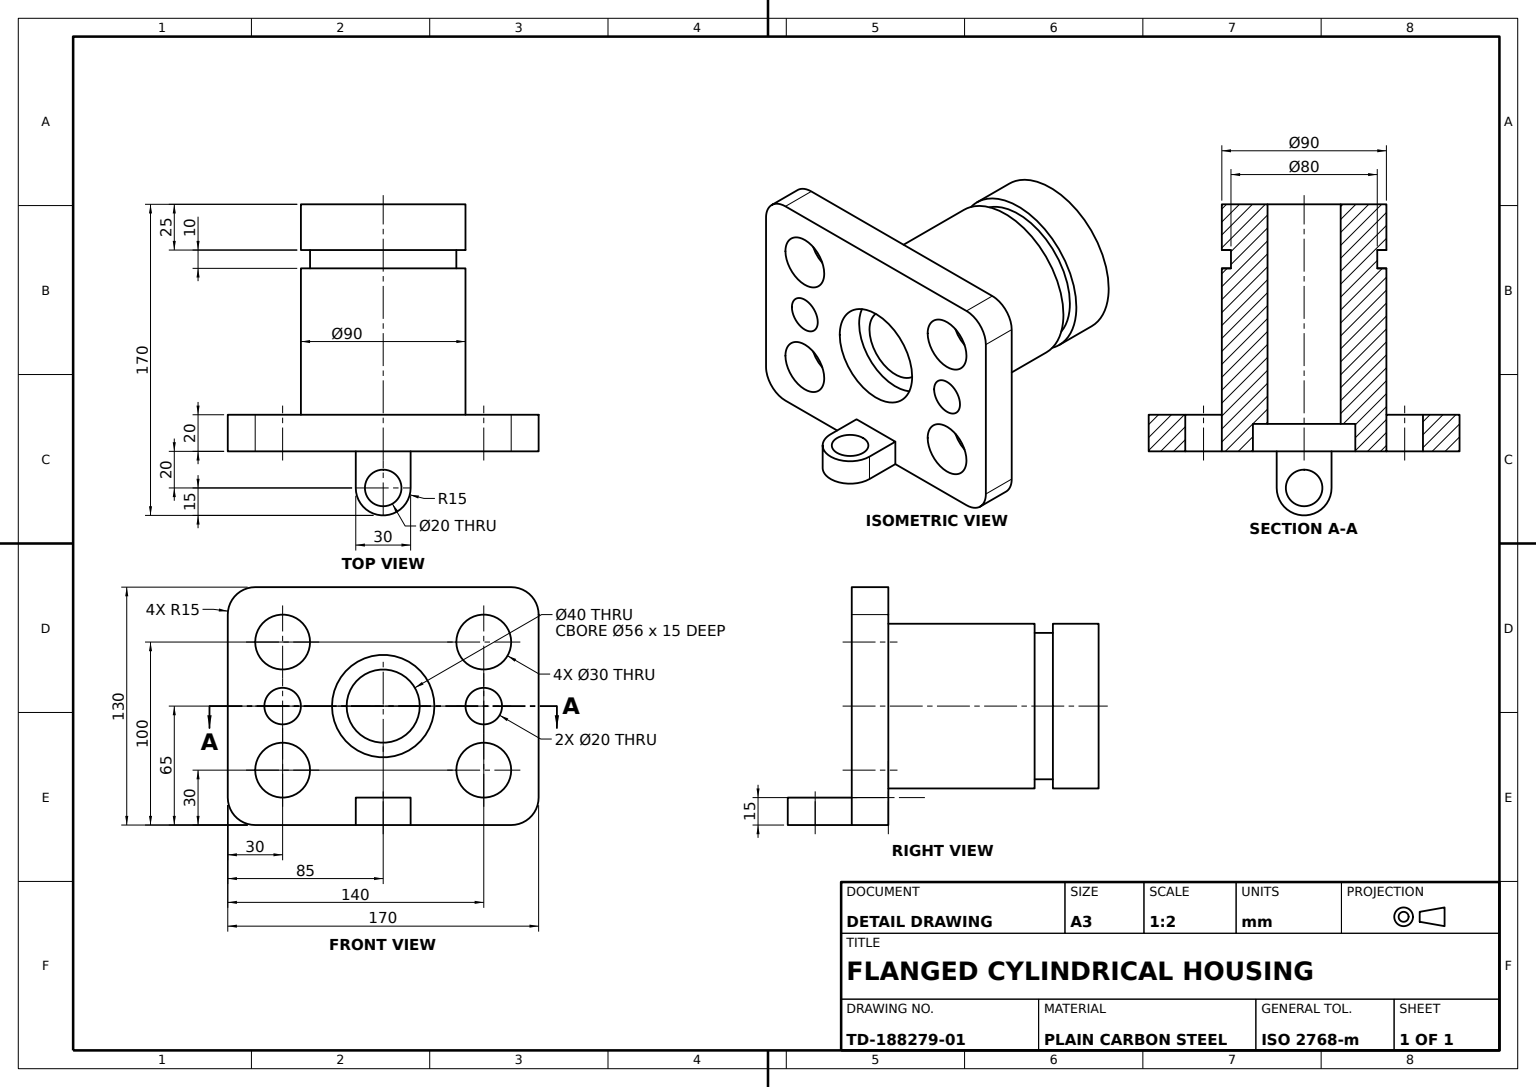
from build123d import *

# Parameters (mm, degrees)
COLUMN_BASE_SKETCH_R    = 45
COLUMN_BASE_90_DEPTH    = 25
GROOVE_NECK_SKETCH_R    = 40
GROOVE_NECK_80_DEPTH    = 10
COLUMN_BODY_SKETCH_R    = 45
COLUMN_BODY_90_DEPTH    = 80
TOP_PLATE_170X130_DEPTH = 20
BORE_STEP_SKETCH_R      = 28
BORE_STEP_28_DEPTH      = 15
COLUMN_BORE_SKETCH_R    = 20
COLUMN_BORE_40_DEPTH    = 150
PLATE_HOLES_SKETCH_R    = 15
PLATE_HOLES_SKETCH_R_2  = 10
PLATE_HOLES_6X_DEPTH    = 150
EYE_LUG_DEPTH           = 15
LUG_HOLE_SKETCH_R       = 10
LUG_HOLE_10_DEPTH       = 15


with BuildPart() as part:
    # Column Base Sketch → Column Base Ø90 (new body)
    with BuildSketch(Plane.XY):
        Circle(COLUMN_BASE_SKETCH_R)
    extrude(amount=COLUMN_BASE_90_DEPTH)

    # Groove Neck Sketch → Groove Neck Ø80 (add)
    with BuildSketch(Plane.XY.offset(25)):
        Circle(GROOVE_NECK_SKETCH_R)
    extrude(amount=GROOVE_NECK_80_DEPTH)

    # Column Body Sketch → Column Body Ø90 (add)
    with BuildSketch(Plane.XY.offset(35)):
        Circle(COLUMN_BODY_SKETCH_R)
    extrude(amount=COLUMN_BODY_90_DEPTH)

    # Top Plate Sketch → Top Plate 170x130 (add)
    with BuildSketch(Plane.XY.offset(115)):
        with BuildLine():
            Line((70, 65), (0, 65))
            Line((0, 65), (-70, 65))
            ThreePointArc((-70, 65), (-80.606601718, 60.606601718), (-85, 50))
            Line((-85, 50), (-85, -50))
            ThreePointArc((-85, -50), (-80.606601718, -60.606601718), (-70, -65))
            Line((-70, -65), (70, -65))
            ThreePointArc((70, -65), (80.606601718, -60.606601718), (85, -50))
            Line((85, -50), (85, 50))
            ThreePointArc((85, 50), (80.606601718, 60.606601718), (70, 65))
        make_face()
    extrude(amount=TOP_PLATE_170X130_DEPTH)

    # Bore Step Sketch → Bore Step Ø28 (cut)
    with BuildSketch(Plane.XY.offset(135)):
        Circle(BORE_STEP_SKETCH_R)
    extrude(amount=-BORE_STEP_28_DEPTH, mode=Mode.SUBTRACT)

    # Column Bore Sketch → Column Bore Ø40 (cut)
    with BuildSketch(Plane.XY.offset(120)):
        Circle(COLUMN_BORE_SKETCH_R)
    extrude(amount=-COLUMN_BORE_40_DEPTH, mode=Mode.SUBTRACT)

    # Plate Holes Sketch → Plate Holes 6x (cut)
    with BuildSketch(Plane.XY.offset(135)):
        with Locations((-55, 35)):
            Circle(PLATE_HOLES_SKETCH_R)
        with Locations((55, 35)):
            Circle(PLATE_HOLES_SKETCH_R)
        with Locations((-55, -35)):
            Circle(PLATE_HOLES_SKETCH_R)
        with Locations((55, -35)):
            Circle(PLATE_HOLES_SKETCH_R)
        with Locations((-55, 0)):
            Circle(PLATE_HOLES_SKETCH_R_2)
        with Locations((55, 0)):
            Circle(PLATE_HOLES_SKETCH_R_2)
    extrude(amount=-PLATE_HOLES_6X_DEPTH, mode=Mode.SUBTRACT)

    # Eye Lug Sketch → Eye Lug (add)
    with BuildSketch(Plane.XZ.offset(65)):
        with BuildLine():
            Line((-15, 135), (15, 135))
            Line((15, 135), (15, 155))
            ThreePointArc((15, 155), (0, 170), (-15, 155))
            Line((-15, 155), (-15, 135))
        make_face()
    extrude(amount=-EYE_LUG_DEPTH)

    # Lug Hole Sketch → Lug Hole Ø10 (cut)
    with BuildSketch(Plane(origin=(0, -50, 0), x_dir=(1, 0, 0), z_dir=(0, 1, 0))):
        with Locations(Location((0, -155, 0), (0, 0, 270))):
            Circle(LUG_HOLE_SKETCH_R)
    extrude(amount=-LUG_HOLE_10_DEPTH, mode=Mode.SUBTRACT)


solid = part.part
